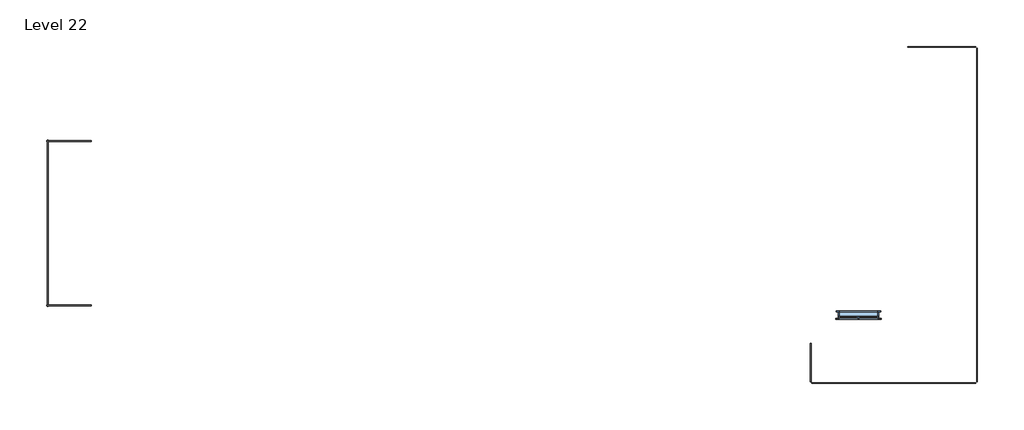
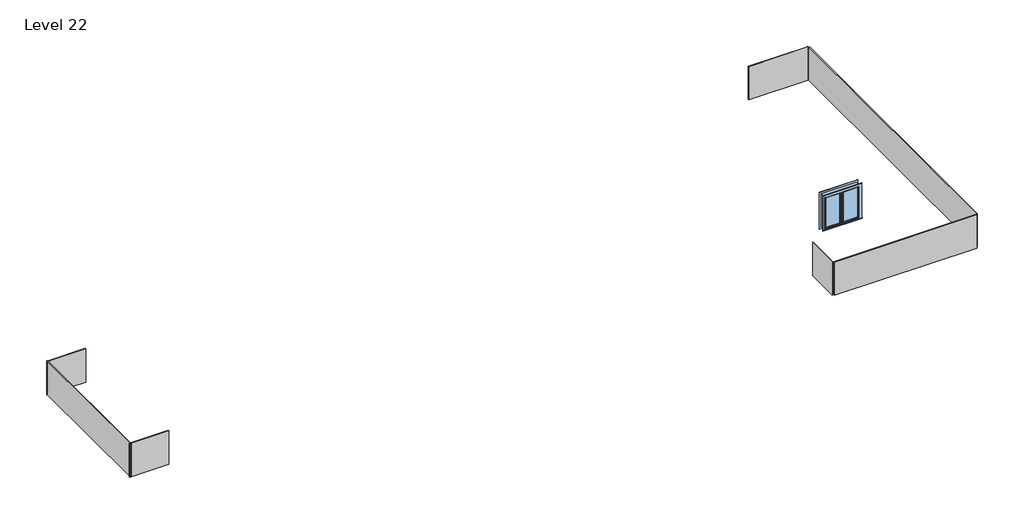
# One storey: 7 plates, 1 window.
"""IFC4 building model written with IfcOpenShell, lengths in millimetres."""

from ifc_helpers import new_model, si_unit, origin, place, context, project, spatial, transform, mapped, element, save
from components import system_panel_glazed_c55d8a5b, system_panel_glazed_07392c36, system_panel_glazed_c10ab47a, system_panel_glazed_5a380d23, system_panel_glazed_51f6397d, system_panel_glazed_4fccefc8, system_panel_glazed_7acd6de3, window_0862ab64

model = new_model("IFC4")

# Units and contexts
model_context = context("Model", 3, world=origin())
ifc_project = project(units=[si_unit("LENGTHUNIT", "METRE", prefix="MILLI")], contexts=[model_context])

# Site, building, storey
site = spatial("IfcSite", under=ifc_project)
building = spatial("IfcBuilding", under=site)
storey = spatial("IfcBuildingStorey", under=building, Name="Level 22", Elevation=35814.0)

# Plates
placement = place(None, origin())
system_panel_glazed_shape = system_panel_glazed_c55d8a5b(model_context)
element("IfcPlate", 1, ObjectType="System Panel : Glazed", at=placement, inside=storey, context=model_context, shape_type="MappedRepresentation", body=[
    mapped(system_panel_glazed_shape, transform((-17978.6550371, -11204.6239591, 35814.0), x_axis=(0.0, -1.0, 0.0), y_axis=(1.0, 0.0, 0.0), z_axis=(0.0, 0.0, 1.0))),
])
system_panel_glazed_2_shape = system_panel_glazed_07392c36(model_context)
element("IfcPlate", 2, ObjectType="System Panel : Glazed", at=placement, inside=storey, context=model_context, shape_type="MappedRepresentation", body=[
    mapped(system_panel_glazed_2_shape, transform((-17302.3800371, -13719.2239591, 35814.0), x_axis=(1.0, 0.0, 0.0), y_axis=(0.0, 1.0, 0.0), z_axis=(0.0, 0.0, 1.0))),
])
system_panel_glazed_3_shape = system_panel_glazed_c10ab47a(model_context)
element("IfcPlate", 3, ObjectType="System Panel : Glazed", at=placement, inside=storey, context=model_context, shape_type="MappedRepresentation", body=[
    mapped(system_panel_glazed_3_shape, transform((-17306.0027899, -8690.0239591, 35814.0), x_axis=(-1.0, 0.0, 0.0), y_axis=(0.0, -1.0, 0.0), z_axis=(0.0, 0.0, 1.0))),
])
system_panel_glazed_4_shape = system_panel_glazed_5a380d23(model_context)
element("IfcPlate", 4, ObjectType="System Panel : Glazed", at=placement, inside=storey, context=model_context, shape_type="MappedRepresentation", body=[
    mapped(system_panel_glazed_4_shape, transform((9019.0964352, -5911.0278294, 35814.0), x_axis=(1.0, 0.0, 0.0), y_axis=(0.0, 1.0, 0.0), z_axis=(0.0, 0.0, 1.0))),
])
system_panel_glazed_5_shape = system_panel_glazed_51f6397d(model_context)
element("IfcPlate", 5, ObjectType="System Panel : Glazed", at=placement, inside=storey, context=model_context, shape_type="MappedRepresentation", body=[
    mapped(system_panel_glazed_5_shape, transform((7571.2964352, -15994.8278294, 35814.0), x_axis=(-1.0, 0.0, 0.0), y_axis=(0.0, -1.0, 0.0), z_axis=(0.0, 0.0, 1.0))),
])
system_panel_glazed_6_shape = system_panel_glazed_4fccefc8(model_context)
element("IfcPlate", 6, ObjectType="System Panel : Glazed", at=placement, inside=storey, context=model_context, shape_type="MappedRepresentation", body=[
    mapped(system_panel_glazed_6_shape, transform((10047.7964352, -10952.9278294, 35814.0), x_axis=(0.0, -1.0, 0.0), y_axis=(1.0, 0.0, 0.0), z_axis=(0.0, 0.0, 1.0))),
])
system_panel_glazed_7_shape = system_panel_glazed_7acd6de3(model_context)
element("IfcPlate", 7, ObjectType="System Panel : Glazed", at=placement, inside=storey, context=model_context, shape_type="MappedRepresentation", body=[
    mapped(system_panel_glazed_7_shape, transform((5094.7964352, -15410.6278294, 35814.0), x_axis=(0.0, 1.0, 0.0), y_axis=(-1.0, 0.0, 0.0), z_axis=(0.0, 0.0, 1.0))),
])

# Window
window_shape = window_0862ab64(model_context)
element("IfcWindow", 8, ObjectType="Casement Dbl with Trim : 48\" x 48\"", at=placement, inside=storey, context=model_context, shape_type="MappedRepresentation", body=[
    mapped(window_shape, transform((6506.0494573, -13957.4308221, 35814.0), x_axis=(-1.0, 0.0, 0.0), y_axis=(0.0, -1.0, 0.0), z_axis=(0.0, 0.0, 1.0))),
])

save(model, "model.ifc")

# Revit data of these elements
# Type "System Panel : Glazed"
#   Construction Type Id = "GSP4R"
#   Analytic Construction = "1/8 in Pilkington single glazing"
#   Visual Light Transmittance = 0.9
#   Solar Heat Gain Coefficient = 0.86
#   Heat Transfer Coefficient (U) = 1.18115 BTU/(h·ft²·°F)
# Type "Casement Dbl with Trim : 48\" x 48\""
#   Type Mark = "10"
#   Construction Type Id = "GSP4R"
#   Assembly Code = "B2020100"
#   Analytic Construction = "1/8 in Pilkington single glazing"
#   Visual Light Transmittance = 0.9
#   Solar Heat Gain Coefficient = 0.78
#   Heat Transfer Coefficient (U) = 0.6496 BTU/(h·ft²·°F)
#   Height = 4' - 0"
#   Default Sill Height = 3' - 0"
#   Trim Projection - Ext. = 0' - 0 1/2"
#   Trim Projection - Int. = 0' - 0 3/4"
#   Trim Width - Exterior = 0' - 3 1/2"
#   Trim Width - Interior = 0' - 3 1/2"
#   Width = 4' - 0"
#   Window Inset = 0' - 0 3/4"
#   Define Thermal Properties by = 1
#   Glass Pane Material = Glass
#   Sash Material = Sash
#   Trim Exterior Material = Trim
#   Trim Interior Material = Trim
#   Wall Closure = (empty or 0)
# Elements 1, 2, 3, 4, 5, 6, 7 (IfcPlate, "System Panel : Glazed")
#   Phase Created = New Construction
#   Materials on its faces: "Glass"
# Element 8 (IfcWindow, "Casement Dbl with Trim : 48\" x 48\"")
#   Mark = "50"
#   Phase Created = New Construction
#   Materials on its faces: "Sash", "Trim", "Glass"
# Materials
#   "Glass": class "Glass", colour RGB 0 128 192, transparency 0.75, Description = "Soda Lime Glass", Cost = 0
#   "Sash": class "Wood", colour RGB 224 178 126, transparency 0
#   "Trim": class "Wood", colour RGB 224 178 126, transparency 0
